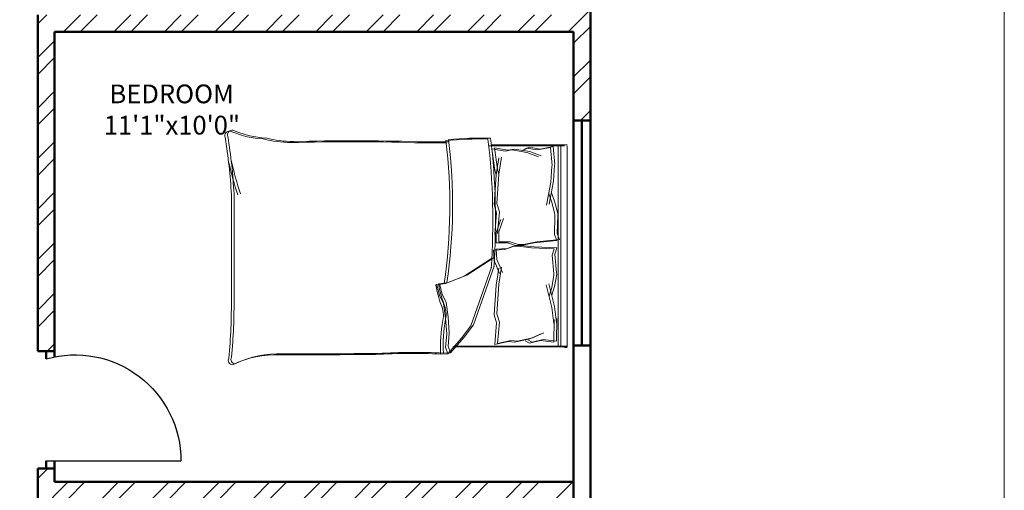
# Model space of a CAD drawing. Units: inches. Extents: x 1901 to 2863, y 888 to 2433.
# Tile 70 of 91: x 2601 to 2863, y 1884 to 2009. Entities that reach past the tile are written whole.
import ezdxf

# ---------------------------------------------------------------- set-up
doc = ezdxf.new("R2010")
doc.units = ezdxf.units.IN
for name, color, linetype, lineweight in [('A-AREA-IDEN', 7, 'Continuous', 18), ('A-DOOR', 4, 'Continuous', 25), ('A-FLOR-FIXT', 9, 'Continuous', 18), ('A-FURN', 8, 'Continuous', 18), ('A-WALL', 7, 'Continuous', 50), ('A-WALL-PATT', 8, 'Continuous', 13)]:
    doc.layers.add(name, color=color, linetype=linetype, lineweight=lineweight)
doc.styles.get("Standard").update_dxf_attribs({"font": 'arial.ttf'})

# ---------------------------------------------------------------- blocks, each defined once
blk = doc.blocks.new('BED-DOUBLE')
for p, q in [((31.18, 59.32), (27.53, 55.16)), ((31.18, 59.32), (27.53, 55.16)), ((31.9, 59.58), (28.25, 55.42)), ((31.9, 59.58), (28.25, 55.42)), ((33.14, 59.41), (31.18, 59.32, 4.35)), ((33.14, 59.41), (31.18, 59.32, 4.35)), ((31.87, 57.59), (31.18, 59.32)), ((31.87, 57.59), (31.18, 59.32)), ((33.85, 59.67), (31.9, 59.58, 4.35)), ((33.85, 59.67), (31.9, 59.58, 4.35)), ((32.59, 57.85), (31.9, 59.58)), ((32.59, 57.85), (31.9, 59.58)), ((32.24, 54.37), (32.59, 57.85)), ((32.24, 54.37), (32.59, 57.85)), ((0.03, 57.78), (0.03, 4.12)), ((0.74, 57.78), (30.62, 57.78)), ((0.74, 57.78), (30.62, 57.78)), ((2.9, 56.23), (2.79, 50.16)), ((2.9, 56.23), (2.79, 50.16)), ((2.9, 56.23), (6.5, 55.8)), ((2.9, 56.23), (6.5, 55.8)), ((3.61, 56.48), (3.51, 50.42)), ((3.61, 56.48), (3.51, 50.42)), ((3.61, 56.48), (7.22, 56.06)), ((3.61, 56.48), (7.22, 56.06)), ((9.3, 55.33), (6.29, 54)), ((9.3, 55.33), (6.29, 54)), ((6.5, 55.8), (9.39, 56.47)), ((6.5, 55.8), (9.39, 56.47)), ((10.01, 55.58), (7.01, 54.26)), ((10.01, 55.58), (7.01, 54.26)), ((7.22, 56.06), (10.11, 56.73)), ((7.22, 56.06), (10.11, 56.73)), ((13.31, 56.23), (9.3, 55.33)), ((13.31, 56.23), (9.3, 55.33)), ((9.39, 56.47), (10.56, 55.89)), ((9.39, 56.47), (10.56, 55.89)), ((14.02, 56.48), (10.01, 55.58)), ((14.02, 56.48), (10.01, 55.58)), ((10.11, 56.73), (11.28, 56.15)), ((10.11, 56.73), (11.28, 56.15)), ((15.11, 56.01), (13.31, 56.23)), ((15.11, 56.01), (13.31, 56.23)), ((15.83, 56.27), (14.02, 56.48)), ((15.83, 56.27), (14.02, 56.48)), ((18.63, 56.89), (15.11, 56.01)), ((18.63, 56.88), (15.11, 56.01)), ((19.35, 57.14), (15.83, 56.27)), ((19.35, 57.14), (15.83, 56.27)), ((18.18, 51.12), (18.63, 56.89)), ((18.18, 51.12), (18.63, 56.88)), ((18.9, 51.38), (19.35, 57.14)), ((18.9, 51.38), (19.35, 57.14)), ((28.25, 55.42), (25.81, 52.11)), ((28.25, 55.42), (25.81, 52.11)), ((31.53, 54.12), (31.87, 57.59)), ((31.53, 54.12), (31.87, 57.59)), ((27.53, 55.16), (25.1, 51.86)), ((27.53, 55.16), (25.1, 51.86)), ((31.87, 49.77), (31.53, 54.12)), ((31.87, 49.77), (31.53, 54.12)), ((32.59, 50.03), (32.24, 54.37)), ((32.59, 50.03), (32.24, 54.37)), ((2.79, 50.16), (2.88, 51.29)), ((2.79, 50.16), (2.88, 51.29)), ((2.88, 51.29), (3.47, 47.02)), ((2.88, 51.29), (3.47, 47.02)), ((3.51, 50.42), (3.6, 51.54)), ((3.51, 50.42), (3.6, 51.54)), ((3.6, 51.54), (4.19, 47.28)), ((3.6, 51.54), (4.19, 47.28)), ((18.81, 48.92), (18.18, 51.12)), ((18.81, 48.92), (18.18, 51.12)), ((19.52, 49.18), (18.9, 51.38)), ((19.52, 49.18), (18.9, 51.38)), ((25.1, 51.86), (22.84, 45.6)), ((25.1, 51.86), (22.84, 45.6)), ((25.81, 52.11), (23.55, 45.85)), ((25.81, 52.11), (23.55, 45.85)), ((33.11, 46.2), (32.59, 50.03)), ((33.11, 46.2), (32.59, 50.03)), ((18.32, 41.05), (18.81, 48.92)), ((18.32, 41.05), (18.81, 48.92)), ((19.04, 41.31), (19.52, 49.18)), ((19.04, 41.31), (19.52, 49.18)), ((32.39, 45.94), (31.87, 49.77)), ((32.39, 45.94), (31.87, 49.77)), ((3.47, 47.02), (4.99, 40.94)), ((3.47, 47.02), (4.99, 40.94)), ((4.19, 47.28), (5.71, 41.19)), ((4.19, 47.28), (5.71, 41.19)), ((22.84, 45.6), (19.54, 36.24)), ((22.84, 45.6), (19.54, 36.24)), ((23.55, 45.85), (20.26, 36.49)), ((23.55, 45.85), (20.26, 36.49)), ((33.44, 43.68), (32.39, 45.94)), ((33.44, 43.68), (32.39, 45.94)), ((34.15, 43.94), (33.11, 46.2)), ((34.15, 43.94), (33.11, 46.2)), ((89.72, 17.13), (89.72, 44.77)), ((89.72, 17.13), (89.72, 44.77)), ((4.15, 43.98), (3.48, 41.66)), ((4.15, 43.98), (3.48, 41.66)), ((4.87, 44.23), (4.2, 41.91)), ((4.87, 44.23), (4.2, 41.91)), ((34.13, 40.9), (33.44, 43.68)), ((34.13, 40.9), (33.44, 43.68)), ((34.85, 41.16), (34.15, 43.94)), ((34.85, 41.16), (34.15, 43.94)), ((89, 16.88), (89, 44.51)), ((89, 16.88), (89, 44.51)), ((3.48, 41.66), (2.87, 38.37)), ((3.48, 41.66), (2.87, 38.37)), ((4.2, 41.91), (3.59, 38.62)), ((4.2, 41.91), (3.59, 38.62)), ((17.57, 36.53), (18.32, 41.05)), ((17.57, 36.52), (18.32, 41.05)), ((18.29, 36.78), (19.04, 41.31)), ((18.29, 36.78), (19.04, 41.31)), ((26.83, 38.64), (31.87, 40.55)), ((26.83, 38.64), (31.87, 40.55)), ((27.55, 38.9), (32.59, 40.81)), ((27.55, 38.9), (32.59, 40.81)), ((31.87, 40.55), (34.13, 40.9)), ((31.87, 40.55), (34.13, 40.9)), ((32.59, 40.81), (34.85, 41.16)), ((32.59, 40.81), (34.85, 41.16)), ((2.87, 38.37), (2.9, 38.01)), ((2.87, 38.37), (2.9, 38.01)), ((2.9, 38.01), (3.37, 33.03)), ((2.9, 38.01), (3.37, 33.04)), ((3.59, 38.62), (3.62, 38.26)), ((3.59, 38.62), (3.62, 38.26)), ((3.62, 38.26), (4.09, 33.29)), ((3.62, 38.26), (4.09, 33.29)), ((18.82, 34.49), (17.38, 37.94)), ((18.82, 34.49), (17.38, 37.94)), ((19.54, 34.74), (18.1, 38.19)), ((19.54, 34.74), (18.1, 38.19)), ((19.54, 33.94), (26.83, 38.64)), ((19.54, 33.94), (26.83, 38.64)), ((20.26, 34.19), (27.55, 38.9)), ((20.26, 34.19), (27.55, 38.9)), ((18.99, 31.73), (18.82, 34.49)), ((18.99, 31.73), (18.82, 34.49)), ((19.71, 31.99), (19.54, 34.74)), ((19.71, 31.99), (19.54, 34.74)), ((3.37, 33.04), (2.82, 31.37)), ((3.37, 33.03), (2.82, 31.37)), ((4.09, 33.29), (3.54, 31.63)), ((4.09, 33.29), (3.54, 31.63)), ((3.54, 31.63), (9.58, 31.36)), ((3.54, 31.63), (9.58, 31.36)), ((13.92, 30.77), (15.99, 31.55)), ((13.92, 30.77), (15.99, 31.55)), ((14.64, 31.02), (16.71, 31.8)), ((14.64, 31.02), (16.71, 31.8)), ((15.99, 31.55), (18.99, 31.73)), ((15.99, 31.55), (18.99, 31.73)), ((16.71, 31.8), (19.71, 31.99)), ((16.71, 31.8), (19.71, 31.99)), ((2.13, 29.14), (8.13, 29.78)), ((2.13, 29.14), (8.13, 29.78)), ((2.78, 27.51), (2.13, 29.14)), ((2.78, 27.51), (2.13, 29.14)), ((2.82, 31.37), (8.86, 31.1)), ((2.82, 31.37), (8.86, 31.1)), ((2.84, 29.39), (8.85, 30.04)), ((2.84, 29.39), (8.85, 30.04)), ((3.49, 27.77), (2.84, 29.39)), ((3.49, 27.77), (2.84, 29.39)), ((8.13, 29.78), (11.7, 30.43)), ((8.13, 29.78), (11.7, 30.43)), ((8.85, 30.04), (12.42, 30.69)), ((8.85, 30.04), (12.42, 30.69)), ((8.86, 31.1), (12.46, 30.68)), ((8.86, 31.1), (12.46, 30.68)), ((9.58, 31.36), (13.18, 30.93)), ((9.58, 31.36), (13.18, 30.93)), ((11.7, 30.43), (13.16, 30.43)), ((11.7, 30.43), (13.16, 30.43)), ((12.42, 30.69), (13.88, 30.69)), ((12.42, 30.69), (13.88, 30.69)), ((12.46, 30.68), (13.92, 30.77)), ((12.46, 30.68), (13.92, 30.77)), ((13.16, 30.43), (15.28, 29.78)), ((13.16, 30.43), (15.28, 29.78)), ((13.18, 30.93), (14.64, 31.02)), ((13.18, 30.93), (14.64, 31.02)), ((13.88, 30.69), (15.99, 30.04)), ((13.88, 30.69), (15.99, 30.04)), ((15.28, 29.78), (18.29, 29.78)), ((15.28, 29.78), (18.29, 29.78)), ((15.99, 30.04), (19, 30.04)), ((15.99, 30.04), (19, 30.04)), ((18.29, 29.78), (18.29, 27.03)), ((18.29, 29.78), (18.29, 27.03)), ((19, 30.04), (19, 27.28)), ((19, 30.04), (19, 27.28)), ((2.61, 22.52), (2.78, 27.51)), ((2.61, 22.52), (2.78, 27.51)), ((3.33, 22.78), (3.49, 27.77)), ((3.33, 22.78), (3.49, 27.77)), ((18.29, 27.03), (17.06, 23.49)), ((18.29, 27.03), (17.06, 23.5)), ((19, 27.28), (17.78, 23.75)), ((19, 27.28), (17.78, 23.75)), ((18.18, 21.73), (18.63, 27.49)), ((18.18, 21.73), (18.63, 27.49)), ((18.9, 21.98), (19.35, 27.75)), ((18.9, 21.98), (19.35, 27.74)), ((2.61, 22.16), (2.61, 22.52)), ((2.61, 22.16), (2.61, 22.52)), ((3.42, 18.91), (2.61, 22.16)), ((3.42, 18.91), (2.61, 22.16)), ((3.33, 22.42), (3.33, 22.78)), ((3.33, 22.42), (3.33, 22.78)), ((4.14, 19.17), (3.33, 22.42)), ((4.14, 19.17), (3.33, 22.42)), ((18.81, 19.53), (18.18, 21.73)), ((18.81, 19.53), (18.18, 21.73)), ((19.52, 19.78), (18.9, 21.98)), ((19.52, 19.78), (18.9, 21.98)), ((4.24, 16.64), (3.42, 18.91)), ((4.24, 16.64), (3.42, 18.91)), ((3.75, 13.56), (4.89, 19.73)), ((3.75, 13.56), (4.89, 19.73)), ((4.95, 16.9), (4.14, 19.17)), ((4.95, 16.9), (4.14, 19.17)), ((4.47, 13.81), (5.6, 19.98)), ((4.47, 13.81), (5.6, 19.98)), ((18.32, 11.66), (18.81, 19.53)), ((18.32, 11.66), (18.81, 19.53)), ((19.04, 11.91), (19.52, 19.78)), ((19.04, 11.91), (19.52, 19.78)), ((3.42, 9.27), (3.75, 13.56)), ((3.42, 9.27), (3.75, 13.56)), ((4.14, 9.52), (4.47, 13.81)), ((4.14, 9.52), (4.47, 13.81)), ((17.57, 7.13), (18.32, 11.66)), ((17.57, 7.13), (18.32, 11.66)), ((18.29, 7.38), (19.04, 11.91)), ((18.29, 7.39), (19.04, 11.91)), ((18.32, 11.66), (18.68, 10.38)), ((18.32, 11.66), (18.68, 10.38)), ((19.04, 11.91), (19.4, 10.64)), ((19.04, 11.91), (19.4, 10.64)), ((19.4, 10.64), (20.21, 4.92)), ((19.4, 10.64), (20.21, 4.92)), ((3.4, 9.15), (3.42, 9.27)), ((3.4, 9.15), (3.42, 9.27)), ((3.77, 4.34), (3.4, 9.15)), ((3.77, 4.34), (3.4, 9.15)), ((4.12, 9.4), (4.14, 9.52)), ((4.12, 9.4), (4.14, 9.52)), ((4.49, 4.6), (4.12, 9.4)), ((4.49, 4.6), (4.12, 9.4)), ((18.68, 10.38), (19.5, 4.66)), ((18.68, 10.38), (19.5, 4.66)), ((10.08, 5.63), (7, 6.77)), ((10.08, 5.63), (7, 6.77)), ((10.8, 5.89), (7.71, 7.03)), ((10.8, 5.89), (7.71, 7.03)), ((14.14, 4.99), (10.08, 5.63)), ((14.14, 4.99), (10.08, 5.63)), ((14.86, 5.24), (10.8, 5.89)), ((14.86, 5.24), (10.8, 5.89)), ((10.96, 4.76), (12.1, 5.4)), ((10.96, 4.75), (12.1, 5.4)), ((15.92, 5.31), (14.14, 4.99)), ((15.92, 5.31), (14.14, 4.99)), ((16.64, 5.57), (14.86, 5.24)), ((16.64, 5.57), (14.86, 5.24)), ((19.5, 4.66), (15.92, 5.31)), ((19.5, 4.66), (15.92, 5.31)), ((20.21, 4.92), (16.64, 5.57)), ((20.21, 4.92), (16.64, 5.57)), ((3.75, 4.34), (7.32, 4.99)), ((3.75, 4.34), (7.32, 4.99)), ((4.47, 4.59), (8.04, 5.24)), ((4.47, 4.59), (8.04, 5.24)), ((7.32, 4.99), (10.24, 4.5)), ((7.32, 4.99), (10.24, 4.5)), ((8.04, 5.24), (10.96, 4.75)), ((8.04, 5.24), (10.96, 4.76)), ((10.24, 4.5), (11.38, 5.15)), ((10.24, 4.5), (11.38, 5.15))]:
    blk.add_line(p, q)
for centre, radius, start, end in [((77.12, 85.47), 25.9, 267.4714, 296.4681), ((77.12, 85.47), 25.9, 267.4714, 296.4681), ((77.84, 85.73), 25.9, 267.4714, 296.4681), ((77.84, 85.73), 25.9, 267.4714, 296.4681), ((88.58, 61.05), 1.24, 332.6588, 86.02), ((88.58, 61.05), 1.24, 332.6588, 86.02), ((238.36, 46.17), 149.37, 174.4998, 180.6351), ((238.36, 46.17), 149.37, 174.4998, 180.6351), ((89.3, 61.31), 1.24, 332.6588, 86.02), ((89.3, 61.31), 1.24, 332.6588, 86.02), ((239.08, 46.42), 149.37, 174.4998, 180.6351), ((239.08, 46.42), 149.37, 174.4998, 180.6351), ((-7.45, 57.59), 40.62, 349.8763, 2.5657), ((-7.45, 57.59), 40.62, 349.8763, 2.5657), ((40.8, 204.6), 145.39, 266.9791, 273.8365), ((40.8, 204.6), 145.39, 266.9791, 273.8365), ((-6.73, 57.85), 40.62, 349.8763, 2.5657), ((-6.73, 57.85), 40.62, 349.8763, 2.5657), ((41.52, 204.86), 145.39, 266.9791, 273.8365), ((41.52, 204.86), 145.39, 266.9791, 273.8365), ((76.17, -5062.23), 5121.82, 90.00217, 90.28689), ((76.17, -5062.23), 5121.82, 90.00217, 90.28689), ((76.89, -5061.97), 5121.82, 90.00217, 90.28689), ((76.89, -5061.97), 5121.82, 90.00217, 90.28689), ((39.4, 49.08), 6.99, 168.6608, 203.7384), ((39.4, 49.08), 6.99, 168.6608, 203.7384), ((40.11, 49.33), 6.99, 168.6608, 203.7384), ((40.11, 49.33), 6.99, 168.6608, 203.7384), ((1.69, 34.94), 33.29, 10.6617, 19.8806), ((1.69, 34.94), 33.29, 10.6617, 19.8806), ((2.41, 35.2), 33.29, 10.6617, 19.8806), ((2.41, 35.2), 33.29, 10.6617, 19.8806), ((175.53, 19.9), 144.86, 171.7845, 186.9006), ((175.53, 19.9), 144.86, 171.7845, 186.9006), ((176.25, 20.16), 144.86, 171.7845, 186.9006), ((176.25, 20.15), 144.86, 171.7845, 186.9006), ((34.2, 41.1), 0.207, 250.2464, 1.1377), ((34.2, 41.1), 0.207, 250.2464, 1.1377), ((34.92, 41.35), 0.207, 250.2464, 1.1377), ((34.92, 41.35), 0.207, 250.2464, 1.1377), ((205.14, 24.2), 185.22, 176.0865, 186.7821), ((205.14, 24.2), 185.22, 176.0865, 186.7821), ((204.43, 23.94), 185.22, 176.0865, 186.7821), ((204.43, 23.94), 185.22, 176.0865, 186.7821), ((225.52, 24.02), 136.7, 182.9958, 189.4091), ((225.52, 24.02), 136.7, 182.9958, 189.4091), ((226.23, 24.28), 136.7, 182.9958, 189.4091), ((226.23, 24.28), 136.7, 182.9958, 189.4091), ((23.31, 95.84), 93.53, 268.7218, 275.604), ((23.31, 95.84), 93.53, 268.7218, 275.604), ((35.03, -187.88), 190.99, 88.4762, 91.0082), ((35.03, -187.88), 190.99, 88.4762, 91.0082), ((35.74, -187.62), 190.99, 88.4762, 91.0082), ((35.74, -187.62), 190.99, 88.4762, 91.0082), ((56.85, 544.3), 541.51, 268.2277, 271.7185), ((56.85, 544.3), 541.51, 268.2277, 271.7185), ((57.57, 544.55), 541.51, 268.2277, 271.7185), ((57.57, 544.55), 541.51, 268.2277, 271.7185), ((72.46, -30.24), 33.27, 76.0648, 88.9113), ((72.46, -30.24), 33.27, 76.0648, 88.9113), ((73.18, -29.98), 33.27, 76.0648, 88.9113), ((73.18, -29.98), 33.27, 76.0648, 88.9113), ((22.59, 95.58), 93.53, 268.7218, 275.604), ((22.59, 95.58), 93.53, 268.7218, 275.604), ((78.93, -24.35), 26.45, 67.9751, 86.652), ((78.93, -24.35), 26.45, 67.9751, 86.652), ((79.65, -24.1), 26.45, 67.9751, 86.652), ((79.65, -24.1), 26.45, 67.9751, 86.652), ((89.53, 1.18), 1.22, 236.1736, 23.4781), ((89.53, 1.18), 1.22, 236.1736, 23.4781), ((90.25, 1.44), 1.22, 236.1736, 23.4781), ((90.25, 1.44), 1.22, 236.1736, 23.4781)]:
    blk.add_arc(centre, radius, start, end)
blk = doc.blocks.new('DOOR-28')
blk.add_line((28.27, 35.98), (28.27, -0.02))
blk.add_arc((28.27, 28.24), 28.25, 164.0861, 270)

msp = doc.modelspace()

# ---------------------------------------------------------------- hatches: boundary and pattern name
at = {"layer": 'A-WALL-PATT'}
h = msp.add_hatch(dxfattribs=at)
h.set_pattern_fill('ANSI32', color=256)
h.paths.add_polyline_path([(2192.5, 2274.13), (2141.26, 2274.13), (2141.26, 2269.63), (2192.5, 2269.63)])
h.paths.add_polyline_path([(2259.93, 2274.13), (2216.5, 2274.13), (2216.5, 2269.63), (2255.43, 2269.63), (2255.43, 2214.63), (2250.81, 2214.63), (2250.81, 2210.13), (2259.93, 2210.13), (2259.93, 2215.13), (2271.76, 2215.13), (2271.76, 2217.38), (2271.76, 2219.63), (2259.93, 2219.63)])
h.paths.add_polyline_path([(2171.43, 2269.63), (2166.93, 2269.63), (2166.93, 2219.63), (2121.24, 2219.63), (2121.24, 2215.13), (2166.93, 2215.13), (2166.93, 2083.13), (2161.81, 2083.13), (2161.81, 2078.63), (2171.43, 2078.63), (2177, 2078.63), (2177, 2080.88), (2177, 2083.13), (2171.43, 2083.13), (2171.43, 2210.13), (2230.91, 2210.13), (2230.91, 2212.38), (2230.91, 2214.63), (2171.43, 2214.63)])
h.paths.add_polyline_path([(2117.26, 2274.13), (2089.43, 2274.13), (2089.43, 2219.63), (2081.14, 2219.63), (2081.14, 2215.13), (2089.43, 2215.13), (2098, 2215.13), (2098, 2217.38), (2098, 2219.63), (2093.93, 2219.63), (2093.93, 2269.63), (2117.26, 2269.63), (2117.26, 2271.88)])
h.paths.add_polyline_path([(2343.43, 2219.63), (2329.29, 2219.63), (2329.29, 2215.13), (2338.93, 2215.13), (2338.93, 2184.74), (2343.43, 2184.74)])
h.paths.add_polyline_path([(2338.93, 2083.13), (2329.29, 2083.13), (2208.97, 2083.13), (2208.97, 2078.63), (2338.93, 2078.63)])
h.paths.add_polyline_path([(2343.43, 2136.74), (2338.93, 2136.74), (2338.93, 1872.63), (2343.43, 1872.63)])
h.paths.add_polyline_path([(2343.43, 1863.63), (2397.68, 1863.63), (2397.68, 1821.63), (2384.14, 1821.63), (2384.14, 1812.63), (2418.33, 1812.63), (2418.33, 1817.13), (2418.33, 1821.63), (2406.68, 1821.63), (2406.68, 1863.63), (2459.5, 1863.63), (2459.5, 1821.63), (2447.14, 1821.63), (2447.14, 1812.63), (2459.5, 1812.63), (2468.5, 1812.63), (2468.5, 1872.63), (2394.43, 1872.63), (2334.43, 1872.63), (2334.43, 1812.63), (2343.43, 1812.63), (2353.25, 1812.63), (2353.25, 1821.63), (2343.43, 1821.63)])
h.paths.add_polyline_path([(2510.01, 1872.63), (2468.5, 1872.63), (2468.5, 1868.13), (2510.01, 1868.13)])
h.paths.add_polyline_path([(2514.01, 1817.13), (2468.5, 1817.13), (2468.5, 1812.63), (2482.11, 1812.63), (2482.11, 1800.61), (2486.61, 1800.61), (2486.61, 1812.63), (2514.01, 1812.63)])
h.paths.add_polyline_path([(2299.25, 1814.88), (2299.25, 1817.13), (2295.93, 1817.13), (2295.93, 1854.17), (2293.68, 1854.17), (2291.43, 1854.17), (2291.43, 1817.13), (2266.11, 1817.13), (2266.11, 1812.63), (2299.25, 1812.63)])
h.paths.add_polyline_path([(2218.11, 1817.13), (2206.46, 1817.13), (2171.43, 1817.13), (2171.43, 1949.13), (2190.1, 1949.13), (2190.1, 1953.63), (2163.47, 1953.63), (2163.47, 1949.13), (2166.93, 1949.13), (2166.93, 1817.13), (2114.3, 1817.13), (2114.3, 1812.63), (2218.11, 1812.63)])
h.paths.add_polyline_path([(2029.43, 1970.92), (2024.93, 1970.92), (2024.93, 1912.72), (2029.43, 1912.72)])
h.paths.add_polyline_path([(2132.3, 1953.63), (2113.93, 1953.63), (2113.93, 1975.89), (2111.68, 1975.89), (2109.43, 1975.89), (2109.43, 1953.63), (2029.43, 1953.63), (2029.43, 1949.13), (2132.3, 1949.13)])
h.paths.add_polyline_path([(2029.43, 1853.61), (2029.31, 1853.61), (2029.31, 1853.61), (2029.43, 1853.61), (2029.43, 1864.72), (2024.93, 1864.72), (2024.93, 1812.63), (2066.3, 1812.63), (2066.3, 1814.88), (2066.3, 1817.13), (2029.43, 1817.13)])
h.paths.add_polyline_path([(2122.93, 2010.09), (2120.68, 2010.09), (2118.43, 2010.09), (2118.43, 2006.13), (2029.43, 2006.13), (2029.43, 2001.63), (2109.43, 2001.63), (2109.43, 1998.04), (2113.93, 1998.04), (2113.93, 2001.63), (2122.93, 2001.63)])
h.paths.add_polyline_path([(2029.43, 2031.38), (2024.93, 2031.38), (2024.93, 1994.92), (2027.18, 1994.92), (2029.43, 1994.92)])
h.paths.add_polyline_path([(2029.43, 2136.74), (2024.93, 2136.74), (2024.93, 2067.38), (2027.18, 2067.38), (2029.43, 2067.38)])
h.paths.add_polyline_path([(2125.62, 2083.13), (2029.43, 2083.13), (2029.43, 2078.63), (2118.43, 2078.63), (2118.43, 2030.71), (2122.93, 2030.71), (2122.93, 2078.63), (2125.62, 2078.63)])
h.paths.add_polyline_path([(2029.43, 2215.13), (2040.47, 2215.13), (2040.47, 2217.38), (2040.47, 2219.63), (2024.93, 2219.63), (2024.93, 2184.74), (2029.43, 2184.74), (2029.43, 2187.78)])
h.paths.add_polyline_path([(2686.43, 2274.13), (2659.28, 2274.13), (2659.28, 2269.63), (2681.93, 2269.63), (2681.93, 2219.63), (2676.82, 2219.63), (2676.82, 2215.13), (2681.93, 2215.13), (2697.01, 2215.13), (2697.01, 2217.38), (2697.01, 2219.63), (2686.43, 2219.63)])
h.paths.add_polyline_path([(2609.93, 2269.63), (2635.28, 2269.63), (2635.28, 2274.13), (2571.43, 2274.13), (2571.43, 2269.63), (2605.43, 2269.63), (2605.43, 2214.63), (2549.1, 2214.63), (2549.1, 2210.13), (2605.43, 2210.13), (2605.43, 2083.13), (2601.01, 2083.13), (2601.01, 2080.88), (2601.01, 2078.63), (2609.93, 2078.63), (2616.16, 2078.63), (2616.16, 2080.88), (2616.16, 2083.13), (2609.93, 2083.13), (2609.93, 2215.13), (2651.46, 2215.13), (2651.46, 2217.38), (2651.46, 2219.63), (2609.93, 2219.63)])
h.paths.add_polyline_path([(2521.43, 2269.63), (2547.43, 2269.63), (2547.43, 2271.88), (2547.43, 2274.13), (2516.93, 2274.13), (2516.93, 2219.63), (2506.41, 2219.63), (2506.41, 2215.13), (2516.93, 2215.13), (2516.93, 2210.13), (2525.4, 2210.13), (2525.4, 2212.38), (2525.4, 2214.63), (2521.43, 2214.63)])
h.paths.add_polyline_path([(2456.01, 2219.63), (2439.43, 2219.63), (2439.43, 2187.89), (2443.93, 2187.89), (2443.93, 2215.13), (2456.01, 2215.13)])
h.paths.add_polyline_path([(2752.93, 2219.63), (2739.48, 2219.63), (2739.48, 2215.13), (2748.43, 2215.13), (2748.43, 2187.89), (2752.93, 2187.89)])
h.paths.add_polyline_path([(2752.93, 2139.89), (2748.43, 2139.89), (2748.43, 2083.13), (2648.42, 2083.13), (2648.42, 2078.63), (2654.93, 2078.63), (2654.93, 2039.44), (2659.43, 2039.44), (2659.43, 2078.63), (2748.43, 2078.63), (2748.43, 2063.43), (2752.93, 2063.43)])
h.paths.add_polyline_path([(2752.93, 2010.63), (2659.43, 2010.63), (2659.43, 2015.65), (2654.93, 2015.65), (2654.93, 2010.63), (2605.43, 2010.63), (2605.43, 1920.97), (2609.93, 1920.97), (2609.93, 2006.13), (2748.43, 2006.13), (2748.43, 1982.47), (2752.93, 1982.47)])
h.paths.add_polyline_path([(2752.93, 2027.43), (2748.43, 2027.43), (2748.43, 2010.63), (2752.93, 2010.63)])
h.paths.add_polyline_path([(2748.43, 1886.13), (2609.93, 1886.13), (2609.93, 1889.72), (2605.43, 1889.72), (2605.43, 1861.26), (2609.93, 1861.26), (2609.93, 1881.63), (2748.43, 1881.63)])
h.paths.add_polyline_path([(2456.86, 2228.83), (2498.4, 2228.83), (2498.4, 2247.49), (2456.86, 2247.49)], flags=9)
h.paths.add_polyline_path([(2038.6, 2237.42), (2080.17, 2237.42), (2080.17, 2256.08), (2038.6, 2256.08)], flags=9)
h.paths.add_polyline_path([(2292.01, 1062.39), (2539.93, 1062.39), (2539.93, 1099.49), (2292.01, 1099.49)], flags=9)
h.paths.add_polyline_path([(2424.91, 1832.25), (2448.51, 1832.25), (2448.51, 1846.68), (2424.91, 1846.68)], flags=25)
h.paths.add_polyline_path([(2359.08, 1832.25), (2382.68, 1832.25), (2382.68, 1846.68), (2359.08, 1846.68)], flags=25)
h.paths.add_polyline_path([(2352.9, 1684.8), (2367.54, 1684.8), (2367.54, 1697.17), (2352.9, 1697.17)], flags=9)
h.paths.add_polyline_path([(2079.29, 1755.83), (2169.02, 1755.83), (2169.02, 1774.37), (2079.29, 1774.37)], flags=9)
h.paths.add_polyline_path([(2404.09, 1373.86), (2404.09, 1463.59), (2385.54, 1463.59), (2385.54, 1373.86)], flags=9)
h.paths.add_polyline_path([(2268.09, 2236.37), (2309.64, 2236.37), (2309.64, 2255.03), (2268.09, 2255.03)], flags=9)
h.paths.add_polyline_path([(2575.96, 1700.95), (2665.7, 1700.95), (2665.7, 1719.5), (2575.96, 1719.5)], flags=9)
h.paths.add_polyline_path([(2302.96, 1878.47), (2329.52, 1878.47), (2329.52, 1888.78), (2302.96, 1888.78)], flags=9)
h.paths.add_polyline_path([(2097.42, 2240.58), (2126.57, 2240.58), (2126.57, 2259.23), (2097.42, 2259.23)], flags=9)
h.paths.add_polyline_path([(2208.72, 2246.12), (2237.88, 2246.12), (2237.88, 2264.78), (2208.72, 2264.78)], flags=9)
h.paths.add_polyline_path([(2038.15, 1925.96), (2076.99, 1925.96), (2076.99, 1944.62), (2038.15, 1944.62)], flags=9)
h.paths.add_polyline_path([(2239.14, 1926.67), (2288.46, 1926.67), (2288.46, 1945.33), (2239.14, 1945.33)], flags=9)
h.paths.add_polyline_path([(2175.43, 2007.33), (2212.36, 2007.33), (2212.36, 2025.99), (2175.43, 2025.99)], flags=9)
h.paths.add_polyline_path([(2225.03, 2091.79), (2263.87, 2091.79), (2263.87, 2110.45), (2225.03, 2110.45)], flags=9)
h.paths.add_polyline_path([(2035.4, 2098.48), (2074.24, 2098.48), (2074.24, 2117.14), (2035.4, 2117.14)], flags=9)
h.paths.add_polyline_path([(2050.1, 2029.21), (2083.26, 2029.21), (2083.26, 2047.87), (2050.1, 2047.87)], flags=9)
h.paths.add_polyline_path([(2069.68, 1956.72), (2098.83, 1956.72), (2098.83, 1975.38), (2069.68, 1975.38)], flags=25)
h.paths.add_polyline_path([(2328.62, 1753.34), (2361.66, 1753.34), (2361.66, 1771.99), (2328.62, 1771.99)], flags=9)
h.paths.add_polyline_path([(2395.16, 2060.89), (2395.16, 2140.65), (2378.68, 2140.65), (2378.68, 2060.89)], flags=9)
h.paths.add_polyline_path([(2463.73, 2059.02), (2492.89, 2059.02), (2492.89, 2077.68), (2463.73, 2077.68)], flags=9)
h.paths.add_polyline_path([(2458.03, 2181.54), (2496.87, 2181.54), (2496.87, 2200.19), (2458.03, 2200.19)], flags=9)
h.paths.add_polyline_path([(2527.58, 2243.07), (2556.73, 2243.07), (2556.73, 2261.73), (2527.58, 2261.73)], flags=9)
h.paths.add_polyline_path([(2694.46, 2232.77), (2736.03, 2232.77), (2736.03, 2251.42), (2694.46, 2251.42)], flags=9)
h.paths.add_polyline_path([(2637.82, 2249.22), (2666.98, 2249.22), (2666.98, 2267.88), (2637.82, 2267.88)], flags=9)
h.paths.add_polyline_path([(2623.69, 2183.54), (2662.53, 2183.54), (2662.53, 2202.2), (2623.69, 2202.2)], flags=9)
h.paths.add_polyline_path([(2691.97, 2021.5), (2725.12, 2021.5), (2725.12, 2040.16), (2691.97, 2040.16)], flags=9)
h.paths.add_polyline_path([(2621.04, 1975.91), (2662.34, 1975.91), (2662.34, 1994.57), (2621.04, 1994.57)], flags=25)
h.paths.add_polyline_path([(2479.03, 1927.62), (2519.84, 1927.62), (2519.84, 1946.28), (2479.03, 1946.28)], flags=9)
h.paths.add_polyline_path([(2670.94, 1849.08), (2716.01, 1849.08), (2716.01, 1867.73), (2670.94, 1867.73)], flags=9)
h.paths.add_polyline_path([(2523.61, 1782.96), (2550.17, 1782.96), (2550.17, 1793.26), (2523.61, 1793.26)], flags=9)
h.paths.add_polyline_path([(2450.84, 1207.33), (2492.39, 1207.33), (2492.39, 1225.99), (2450.84, 1225.99)], flags=9)
h.paths.add_polyline_path([(2527.75, 1203.84), (2556.91, 1203.84), (2556.91, 1222.5), (2527.75, 1222.5)], flags=9)
h.paths.add_polyline_path([(2639.11, 1207.2), (2668.27, 1207.2), (2668.27, 1225.86), (2639.11, 1225.86)], flags=9)
h.paths.add_polyline_path([(2692.59, 1218.97), (2734.17, 1218.97), (2734.17, 1237.62), (2692.59, 1237.62)], flags=9)
h.paths.add_polyline_path([(2669.27, 1366.33), (2708.11, 1366.33), (2708.11, 1384.99), (2669.27, 1384.99)], flags=9)
h.paths.add_polyline_path([(2463.31, 1358.03), (2502.15, 1358.03), (2502.15, 1376.69), (2463.31, 1376.69)], flags=9)
h.paths.add_polyline_path([(2494.72, 1449.96), (2531.65, 1449.96), (2531.65, 1468.62), (2494.72, 1468.62)], flags=9)
h.paths.add_polyline_path([(2675.57, 1422.16), (2708.72, 1422.16), (2708.72, 1440.81), (2675.57, 1440.81)], flags=9)
h.paths.add_polyline_path([(2685.63, 1493.89), (2714.79, 1493.89), (2714.79, 1512.55), (2685.63, 1512.55)], flags=9)
h.paths.add_polyline_path([(2686.8, 1529.91), (2725.65, 1529.91), (2725.65, 1548.57), (2686.8, 1548.57)], flags=9)
h.paths.add_polyline_path([(2503.65, 1537.99), (2552.97, 1537.99), (2552.97, 1556.65), (2503.65, 1556.65)], flags=9)
h.paths.add_polyline_path([(2291.71, 1643.5), (2318.28, 1643.5), (2318.28, 1653.81), (2291.71, 1653.81)], flags=9)
h.paths.add_polyline_path([(2450.63, 1610.52), (2477.19, 1610.52), (2477.19, 1620.82), (2450.63, 1620.82)], flags=9)
h.paths.add_polyline_path([(2359.99, 1551.81), (2422.25, 1551.81), (2422.25, 1562.12), (2359.99, 1562.12)], flags=9)
h.paths.add_polyline_path([(2280.11, 1249.01), (2321.65, 1249.01), (2321.65, 1267.66), (2280.11, 1267.66)], flags=9)
h.paths.add_polyline_path([(2164.06, 1274.23), (2193.22, 1274.23), (2193.22, 1292.89), (2164.06, 1292.89)], flags=9)
h.paths.add_polyline_path([(2118.21, 1277.69), (2151.25, 1277.69), (2151.25, 1296.35), (2118.21, 1296.35)], flags=9)
h.paths.add_polyline_path([(2031.95, 1268.53), (2073.52, 1268.53), (2073.52, 1287.19), (2031.95, 1287.19)], flags=9)
h.paths.add_polyline_path([(2050.2, 1409.08), (2089.04, 1409.08), (2089.04, 1427.74), (2050.2, 1427.74)], flags=9)
h.paths.add_polyline_path([(2243.74, 1421.03), (2282.58, 1421.03), (2282.58, 1439.69), (2243.74, 1439.69)], flags=9)
h.paths.add_polyline_path([(2190.75, 1509.77), (2231.56, 1509.77), (2231.56, 1528.43), (2190.75, 1528.43)], flags=9)
h.paths.add_polyline_path([(2058.39, 1475.42), (2091.55, 1475.42), (2091.55, 1494.07), (2058.39, 1494.07)], flags=9)
h.paths.add_polyline_path([(2062.45, 1553.09), (2091.6, 1553.09), (2091.6, 1571.75), (2062.45, 1571.75)], flags=9)
h.paths.add_polyline_path([(2219.52, 1590.37), (2266.15, 1590.37), (2266.15, 1609.02), (2219.52, 1609.02)], flags=9)
h.paths.add_polyline_path([(2041.07, 1584.19), (2079.91, 1584.19), (2079.91, 1602.85), (2041.07, 1602.85)], flags=9)
h = msp.add_hatch(dxfattribs=at)
h.set_pattern_fill('ANSI32', color=256)
h.paths.add_polyline_path([(2443.93, 2139.89), (2439.43, 2139.89), (2439.43, 2069.35), (2441.68, 2069.35), (2443.93, 2069.35), (2443.93, 2078.63), (2521.93, 2078.63), (2521.93, 2075.07), (2524.18, 2075.07), (2526.43, 2075.07), (2526.43, 2078.63), (2571.75, 2078.63), (2571.75, 2080.88), (2571.75, 2083.13), (2443.93, 2083.13)])
h.paths.add_polyline_path([(2526.43, 2054.63), (2524.18, 2054.63), (2521.93, 2054.63), (2521.93, 2030.63), (2443.93, 2030.63), (2443.93, 2045.35), (2439.43, 2045.35), (2439.43, 1983.87), (2443.93, 1983.87), (2443.93, 2026.13), (2521.93, 2026.13), (2526.43, 2026.13)])
h.paths.add_polyline_path([(2443.93, 1923.87), (2439.43, 1923.87), (2439.43, 1872.63), (2443.93, 1872.63)])
h.paths.add_polyline_path([(2636.23, 1766.13), (2609.93, 1766.13), (2609.93, 1779.79), (2605.43, 1779.79), (2605.43, 1766.13), (2486.61, 1766.13), (2486.61, 1770.67), (2482.11, 1770.67), (2482.11, 1766.13), (2482.11, 1761.63), (2636.23, 1761.63), (2636.23, 1763.88)])
h.paths.add_polyline_path([(2519.54, 1663.38), (2519.54, 1665.63), (2494.93, 1665.63), (2481.83, 1665.63), (2481.83, 1663.38), (2481.83, 1661.13), (2490.43, 1661.13), (2490.43, 1640.16), (2494.93, 1640.16), (2494.93, 1661.13), (2519.54, 1661.13)])
h.paths.add_polyline_path([(2443.93, 1712.13), (2443.93, 1716.63), (2414.46, 1716.63), (2414.46, 1712.13), (2439.43, 1712.13), (2439.43, 1545.51), (2443.93, 1545.51), (2443.93, 1661.13), (2448.47, 1661.13), (2448.47, 1665.63), (2443.93, 1665.63)])
h.paths.add_polyline_path([(2343.43, 1712.13), (2365.52, 1712.13), (2365.52, 1714.38), (2365.52, 1716.63), (2333.87, 1716.63), (2333.87, 1714.38), (2333.87, 1712.13), (2338.93, 1712.13), (2338.93, 1575.63), (2338.93, 1545.51), (2343.43, 1545.51), (2343.43, 1547.51), (2343.43, 1580.13)])
h.paths.add_polyline_path([(2752.93, 1665.63), (2579.54, 1665.63), (2579.54, 1661.13), (2615.93, 1661.13), (2615.93, 1529.13), (2598.93, 1529.13), (2598.93, 1524.63), (2623.13, 1524.63), (2623.13, 1526.88), (2623.13, 1529.13), (2620.43, 1529.13), (2620.43, 1661.13), (2748.43, 1661.13), (2748.43, 1633.5), (2752.93, 1633.5)])
h.paths.add_polyline_path([(2752.93, 1419.93), (2748.43, 1419.93), (2748.43, 1400.13), (2659.43, 1400.13), (2659.43, 1444.33), (2657.18, 1444.33), (2654.93, 1444.33), (2654.93, 1400.13), (2643.65, 1400.13), (2643.65, 1395.63), (2748.43, 1395.63), (2748.43, 1364.04), (2752.93, 1364.04)])
h.paths.add_polyline_path([(2752.93, 1492.88), (2748.43, 1492.88), (2748.43, 1476.63), (2667.43, 1476.63), (2667.43, 1479.71), (2665.18, 1479.71), (2662.93, 1479.71), (2662.93, 1476.63), (2654.93, 1476.63), (2654.93, 1469.54), (2659.43, 1469.54), (2659.43, 1472.13), (2748.43, 1472.13), (2748.43, 1455.93), (2752.93, 1455.93)])
h.paths.add_polyline_path([(2752.93, 1304.04), (2748.43, 1304.04), (2748.43, 1263.63), (2738.66, 1263.63), (2738.66, 1259.13), (2752.93, 1259.13)])
h.paths.add_polyline_path([(2685.93, 1259.13), (2695.49, 1259.13), (2695.49, 1261.38), (2695.49, 1263.63), (2677.84, 1263.63), (2677.84, 1261.38), (2677.84, 1259.13), (2681.43, 1259.13), (2681.43, 1203.63), (2653.28, 1203.63), (2653.28, 1199.13), (2685.93, 1199.13), (2685.93, 1203.63)])
h.paths.add_polyline_path([(2609.43, 1395.63), (2611.85, 1395.63), (2611.85, 1400.13), (2598.89, 1400.13), (2598.89, 1397.88), (2598.89, 1395.63), (2604.93, 1395.63), (2604.93, 1268.13), (2554.73, 1268.13), (2554.73, 1265.88), (2554.73, 1263.63), (2604.93, 1263.63), (2604.93, 1203.63), (2571.31, 1203.63), (2571.31, 1199.13), (2604.93, 1199.13), (2629.28, 1199.13), (2629.28, 1201.38), (2629.28, 1203.63), (2609.43, 1203.63), (2609.43, 1258.63), (2609.43, 1259.13), (2654.8, 1259.13), (2654.8, 1263.63), (2609.43, 1263.63)])
h.paths.add_polyline_path([(2443.93, 1304.04), (2439.43, 1304.04), (2439.43, 1259.13), (2443.93, 1259.13), (2456.16, 1259.13), (2456.16, 1261.38), (2456.16, 1263.63), (2443.93, 1263.63)])
h.paths.add_polyline_path([(2525.43, 1263.63), (2531.78, 1263.63), (2531.78, 1268.13), (2520.93, 1268.13), (2520.93, 1263.63), (2511.41, 1263.63), (2511.41, 1259.13), (2520.93, 1259.13), (2520.93, 1199.13), (2547.31, 1199.13), (2547.31, 1201.38), (2547.31, 1203.63), (2525.43, 1203.63)])
h.paths.add_polyline_path([(2443.93, 1434.84), (2439.43, 1434.84), (2439.43, 1364.04), (2441.68, 1364.04), (2443.93, 1364.04)])
h.paths.add_polyline_path([(2567.13, 1400.13), (2443.93, 1400.13), (2443.93, 1395.63), (2567.13, 1395.63)])
h.paths.add_polyline_path([(2443.93, 1545.51), (2439.43, 1545.51), (2439.43, 1494.84), (2443.93, 1494.84)])
h.paths.add_polyline_path([(2494.93, 1553.35), (2492.68, 1553.35), (2490.43, 1553.35), (2490.43, 1524.63), (2494.93, 1524.63), (2525.94, 1524.63), (2525.94, 1526.88), (2525.94, 1529.13), (2494.93, 1529.13)])
h.paths.add_polyline_path([(2752.93, 1573.5), (2748.43, 1573.5), (2748.43, 1529.13), (2657.76, 1529.13), (2657.76, 1524.63), (2662.93, 1524.63), (2662.93, 1498.63), (2667.43, 1498.63), (2667.43, 1524.63), (2748.43, 1524.63), (2748.43, 1516.88), (2752.93, 1516.88)])
h.paths.add_polyline_path([(2038.6, 2237.42), (2080.17, 2237.42), (2080.17, 2256.08), (2038.6, 2256.08)], flags=9)
h.paths.add_polyline_path([(2292.01, 1062.39), (2539.93, 1062.39), (2539.93, 1099.49), (2292.01, 1099.49)], flags=9)
h.paths.add_polyline_path([(2424.91, 1832.25), (2448.51, 1832.25), (2448.51, 1846.68), (2424.91, 1846.68)], flags=9)
h.paths.add_polyline_path([(2359.08, 1832.25), (2382.68, 1832.25), (2382.68, 1846.68), (2359.08, 1846.68)], flags=9)
h.paths.add_polyline_path([(2352.9, 1684.8), (2367.54, 1684.8), (2367.54, 1697.17), (2352.9, 1697.17)], flags=9)
h.paths.add_polyline_path([(2079.29, 1755.83), (2169.02, 1755.83), (2169.02, 1774.37), (2079.29, 1774.37)], flags=9)
h.paths.add_polyline_path([(2404.09, 1373.86), (2404.09, 1463.59), (2385.54, 1463.59), (2385.54, 1373.86)], flags=9)
h.paths.add_polyline_path([(2268.09, 2236.37), (2309.64, 2236.37), (2309.64, 2255.03), (2268.09, 2255.03)], flags=9)
h.paths.add_polyline_path([(2575.96, 1700.95), (2665.7, 1700.95), (2665.7, 1719.5), (2575.96, 1719.5)], flags=9)
h.paths.add_polyline_path([(2302.96, 1878.47), (2329.52, 1878.47), (2329.52, 1888.78), (2302.96, 1888.78)], flags=9)
h.paths.add_polyline_path([(2097.42, 2240.58), (2126.57, 2240.58), (2126.57, 2259.23), (2097.42, 2259.23)], flags=9)
h.paths.add_polyline_path([(2208.72, 2246.12), (2237.88, 2246.12), (2237.88, 2264.78), (2208.72, 2264.78)], flags=9)
h.paths.add_polyline_path([(2038.15, 1925.96), (2076.99, 1925.96), (2076.99, 1944.62), (2038.15, 1944.62)], flags=9)
h.paths.add_polyline_path([(2239.14, 1926.67), (2288.46, 1926.67), (2288.46, 1945.33), (2239.14, 1945.33)], flags=9)
h.paths.add_polyline_path([(2175.43, 2007.33), (2212.36, 2007.33), (2212.36, 2025.99), (2175.43, 2025.99)], flags=9)
h.paths.add_polyline_path([(2225.03, 2091.79), (2263.87, 2091.79), (2263.87, 2110.45), (2225.03, 2110.45)], flags=9)
h.paths.add_polyline_path([(2035.4, 2098.48), (2074.24, 2098.48), (2074.24, 2117.14), (2035.4, 2117.14)], flags=9)
h.paths.add_polyline_path([(2050.1, 2029.21), (2083.26, 2029.21), (2083.26, 2047.87), (2050.1, 2047.87)], flags=9)
h.paths.add_polyline_path([(2069.68, 1956.72), (2098.83, 1956.72), (2098.83, 1975.38), (2069.68, 1975.38)], flags=9)
h.paths.add_polyline_path([(2328.62, 1753.34), (2361.66, 1753.34), (2361.66, 1771.99), (2328.62, 1771.99)], flags=9)
h.paths.add_polyline_path([(2395.16, 2060.89), (2395.16, 2140.65), (2378.68, 2140.65), (2378.68, 2060.89)], flags=9)
h.paths.add_polyline_path([(2463.73, 2059.02), (2492.89, 2059.02), (2492.89, 2077.68), (2463.73, 2077.68)], flags=9)
h.paths.add_polyline_path([(2458.03, 2181.54), (2496.87, 2181.54), (2496.87, 2200.19), (2458.03, 2200.19)], flags=9)
h.paths.add_polyline_path([(2456.86, 2228.83), (2498.4, 2228.83), (2498.4, 2247.49), (2456.86, 2247.49)], flags=9)
h.paths.add_polyline_path([(2527.58, 2243.07), (2556.73, 2243.07), (2556.73, 2261.73), (2527.58, 2261.73)], flags=9)
h.paths.add_polyline_path([(2694.46, 2232.77), (2736.03, 2232.77), (2736.03, 2251.42), (2694.46, 2251.42)], flags=9)
h.paths.add_polyline_path([(2637.82, 2249.22), (2666.98, 2249.22), (2666.98, 2267.88), (2637.82, 2267.88)], flags=9)
h.paths.add_polyline_path([(2623.69, 2183.54), (2662.53, 2183.54), (2662.53, 2202.2), (2623.69, 2202.2)], flags=9)
h.paths.add_polyline_path([(2691.97, 2021.5), (2725.12, 2021.5), (2725.12, 2040.16), (2691.97, 2040.16)], flags=9)
h.paths.add_polyline_path([(2621.04, 1975.91), (2662.34, 1975.91), (2662.34, 1994.57), (2621.04, 1994.57)], flags=9)
h.paths.add_polyline_path([(2479.03, 1927.62), (2519.84, 1927.62), (2519.84, 1946.28), (2479.03, 1946.28)], flags=9)
h.paths.add_polyline_path([(2670.94, 1849.08), (2716.01, 1849.08), (2716.01, 1867.73), (2670.94, 1867.73)], flags=9)
h.paths.add_polyline_path([(2523.61, 1782.96), (2550.17, 1782.96), (2550.17, 1793.26), (2523.61, 1793.26)], flags=9)
h.paths.add_polyline_path([(2450.84, 1207.33), (2492.39, 1207.33), (2492.39, 1225.99), (2450.84, 1225.99)], flags=9)
h.paths.add_polyline_path([(2527.75, 1203.84), (2556.91, 1203.84), (2556.91, 1222.5), (2527.75, 1222.5)], flags=9)
h.paths.add_polyline_path([(2639.11, 1207.2), (2668.27, 1207.2), (2668.27, 1225.86), (2639.11, 1225.86)], flags=9)
h.paths.add_polyline_path([(2692.59, 1218.97), (2734.17, 1218.97), (2734.17, 1237.62), (2692.59, 1237.62)], flags=9)
h.paths.add_polyline_path([(2669.27, 1366.33), (2708.11, 1366.33), (2708.11, 1384.99), (2669.27, 1384.99)], flags=25)
h.paths.add_polyline_path([(2463.31, 1358.03), (2502.15, 1358.03), (2502.15, 1376.69), (2463.31, 1376.69)], flags=9)
h.paths.add_polyline_path([(2494.72, 1449.96), (2531.65, 1449.96), (2531.65, 1468.62), (2494.72, 1468.62)], flags=9)
h.paths.add_polyline_path([(2675.57, 1422.16), (2708.72, 1422.16), (2708.72, 1440.81), (2675.57, 1440.81)], flags=25)
h.paths.add_polyline_path([(2685.63, 1493.89), (2714.79, 1493.89), (2714.79, 1512.55), (2685.63, 1512.55)], flags=9)
h.paths.add_polyline_path([(2686.8, 1529.91), (2725.65, 1529.91), (2725.65, 1548.57), (2686.8, 1548.57)], flags=25)
h.paths.add_polyline_path([(2503.65, 1537.99), (2552.97, 1537.99), (2552.97, 1556.65), (2503.65, 1556.65)], flags=9)
h.paths.add_polyline_path([(2291.71, 1643.5), (2318.28, 1643.5), (2318.28, 1653.81), (2291.71, 1653.81)], flags=9)
h.paths.add_polyline_path([(2450.63, 1610.52), (2477.19, 1610.52), (2477.19, 1620.82), (2450.63, 1620.82)], flags=9)
h.paths.add_polyline_path([(2359.99, 1551.81), (2422.25, 1551.81), (2422.25, 1562.12), (2359.99, 1562.12)], flags=9)
h.paths.add_polyline_path([(2280.11, 1249.01), (2321.65, 1249.01), (2321.65, 1267.66), (2280.11, 1267.66)], flags=9)
h.paths.add_polyline_path([(2164.06, 1274.23), (2193.22, 1274.23), (2193.22, 1292.89), (2164.06, 1292.89)], flags=9)
h.paths.add_polyline_path([(2118.21, 1277.69), (2151.25, 1277.69), (2151.25, 1296.35), (2118.21, 1296.35)], flags=9)
h.paths.add_polyline_path([(2031.95, 1268.53), (2073.52, 1268.53), (2073.52, 1287.19), (2031.95, 1287.19)], flags=9)
h.paths.add_polyline_path([(2050.2, 1409.08), (2089.04, 1409.08), (2089.04, 1427.74), (2050.2, 1427.74)], flags=9)
h.paths.add_polyline_path([(2243.74, 1421.03), (2282.58, 1421.03), (2282.58, 1439.69), (2243.74, 1439.69)], flags=9)
h.paths.add_polyline_path([(2190.75, 1509.77), (2231.56, 1509.77), (2231.56, 1528.43), (2190.75, 1528.43)], flags=9)
h.paths.add_polyline_path([(2058.39, 1475.42), (2091.55, 1475.42), (2091.55, 1494.07), (2058.39, 1494.07)], flags=9)
h.paths.add_polyline_path([(2062.45, 1553.09), (2091.6, 1553.09), (2091.6, 1571.75), (2062.45, 1571.75)], flags=9)
h.paths.add_polyline_path([(2219.52, 1590.37), (2266.15, 1590.37), (2266.15, 1609.02), (2219.52, 1609.02)], flags=9)
h.paths.add_polyline_path([(2041.07, 1584.19), (2079.91, 1584.19), (2079.91, 1602.85), (2041.07, 1602.85)], flags=9)

# ---------------------------------------------------------------- linework, layer by layer
at = {"layer": 'A-FLOR-FIXT'}
msp.add_lwpolyline([(1901.45, 2433.12), (2863.43, 2433.12), (2863.43, 961.82), (1901.45, 961.82)], close=True, dxfattribs=at)
at = {"layer": 'A-FURN'}
for p, q in [((2725.74, 1975.75), (2746.07, 1975.75)), ((2725.74, 1975.75), (2746.07, 1975.75)), ((2726.46, 1976), (2746.79, 1976)), ((2726.46, 1976), (2746.79, 1976)), ((2744.35, 1975.75), (2744.35, 1922.09)), ((2744.35, 1975.75), (2744.35, 1922.09)), ((2745.07, 1976), (2745.07, 1922.35)), ((2745.07, 1976), (2745.07, 1922.35)), ((2746.79, 1922.35), (2716.91, 1922.35)), ((2746.79, 1922.35), (2716.91, 1922.35))]:
    msp.add_line(p, q, dxfattribs=at)
for centre in [(2772.7, 1998.98), (2772.7, 1998.98), (2773.41, 1999.24), (2773.41, 1999.24)]:
    msp.add_arc(centre, 119.53, 193.3832, 197.7053, dxfattribs=at)
at = {"layer": 'A-WALL'}
for p, q in [((2752.93, 2219.63), (2752.93, 1812.63)), ((2605.43, 2010.63), (2605.43, 1920.97)), ((2609.93, 2006.13), (2609.93, 1919.5)), ((2609.93, 2006.13), (2748.43, 2006.13)), ((2748.43, 2006.13), (2748.43, 1817.13)), ((2748.43, 1982.47), (2752.93, 1982.47)), ((2752.93, 1982.47), (2750.68, 1982.47)), ((2750.68, 1982.47), (2750.68, 1934.47)), ((2750.68, 1934.47), (2750.68, 1922.47)), ((2746.79, 1922.09), (2746.07, 1922.09)), ((2752.93, 1922.47), (2748.43, 1922.47)), ((2750.68, 1922.47), (2752.93, 1922.47)), ((2605.43, 1920.97), (2609.93, 1920.97)), ((2609.93, 1920.97), (2607.68, 1920.97)), ((2607.68, 1920.97), (2607.68, 1918.97)), ((2607.68, 1889.72), (2607.68, 1891.72)), ((2609.93, 1891.72), (2609.93, 1886.13)), ((2609.93, 1889.72), (2605.43, 1889.72)), ((2605.43, 1889.72), (2607.68, 1889.72)), ((2605.43, 1889.72), (2605.43, 1861.26)), ((2609.93, 1886.13), (2748.43, 1886.13))]:
    msp.add_line(p, q, dxfattribs=at)

# ---------------------------------------------------------------- block references
at = {"layer": 'A-DOOR', "extrusion": (0, 0, -1), "zscale": -1, "rotation": 270.0987893838629}
msp.add_blockref('DOOR-28', (-2643.69, 1919.97), dxfattribs=at)
at = {"layer": 'A-FURN', "rotation": 180}
msp.add_blockref('BED-DOUBLE', (2746.82, 1979.87), dxfattribs=at)

# ---------------------------------------------------------------- texts
at = {"layer": 'A-AREA-IDEN', "insert": (2623.05, 1992.08), "char_height": 5, "attachment_point": 1}
msp.add_mtext_dynamic_manual_height_columns(' BEDROOM\\P11\'1"x10\'0"', width=176.4178, gutter_width=12.5, heights=[0], dxfattribs=at)

doc.saveas('drawing.dxf')
